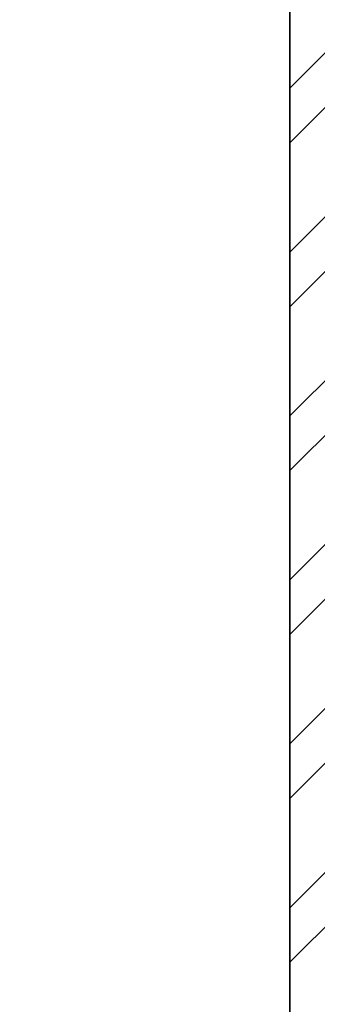
# Model space of a CAD drawing. Units: inches. Extents: x 2168 to 3056, y 1130 to 2629.
# Tile 30 of 42: x 2574 to 2598, y 2305 to 2386. Entities that reach past the tile are written whole.
import ezdxf

# ---------------------------------------------------------------- set-up
doc = ezdxf.new("R2010")
doc.units = ezdxf.units.IN
doc.layers.add('A-WALL', color=7, linetype='Continuous', lineweight=35)
doc.layers.add('A-WALL-PATT', color=143, linetype='Continuous', lineweight=13, true_color=0x7aafdf)

msp = doc.modelspace()

# ---------------------------------------------------------------- hatches: boundary and pattern name
at = {"layer": 'A-WALL-PATT'}
h = msp.add_hatch(dxfattribs=at)
h.set_pattern_fill('ANSI32', color=256)
h.paths.add_polyline_path([(2463.796, 2409.389), (2467.387, 2409.389), (2467.387, 2413.889), (2454.768, 2413.889), (2454.768, 2411.639), (2454.768, 2409.389), (2459.296, 2409.389), (2459.296, 2265.389), (2455.644, 2265.389), (2455.644, 2260.889), (2467.349, 2260.889), (2467.349, 2263.139), (2467.349, 2265.389), (2463.796, 2265.389)])
h.paths.add_polyline_path([(2431.596, 2413.889), (2409.647, 2413.889), (2409.647, 2409.389), (2431.596, 2409.389), (2431.596, 2411.639)])
h.paths.add_polyline_path([(2349.647, 2413.889), (2331.796, 2413.889), (2331.796, 2362.671), (2336.296, 2362.671), (2336.296, 2409.389), (2349.647, 2409.389), (2349.647, 2411.639)])
h.paths.add_polyline_path([(2634.149, 2411.639), (2634.149, 2413.889), (2562.293, 2413.889), (2562.293, 2409.389), (2595.796, 2409.389), (2595.796, 2280.309), (2595.826, 2280.309), (2595.826, 2265.389), (2499.91, 2265.389), (2499.91, 2260.889), (2550.796, 2260.889), (2550.796, 2117.308), (2555.296, 2117.308), (2555.296, 2168.08), (2571.93, 2168.08), (2571.93, 2176.889), (2559.796, 2176.889), (2559.796, 2256.389), (2640.796, 2256.389), (2640.796, 2176.889), (2626.428, 2176.889), (2626.428, 2168.08), (2645.296, 2168.08), (2645.296, 2116.637), (2649.796, 2116.637), (2649.796, 2260.889), (2691.251, 2260.889), (2691.251, 2263.139), (2691.251, 2265.389), (2670.655, 2265.389), (2670.655, 2265.365), (2600.296, 2265.365), (2600.296, 2280.258), (2600.296, 2409.389), (2634.149, 2409.389)])
h.paths.add_polyline_path([(2600.296, 2473.889), (2612.84, 2473.889), (2612.84, 2478.389), (2572.636, 2478.389), (2572.636, 2473.889), (2595.796, 2473.889), (2595.796, 2413.889), (2600.296, 2413.889)])
h.paths.add_polyline_path([(2535.796, 2473.889), (2548.636, 2473.889), (2548.636, 2478.389), (2531.396, 2478.389), (2531.396, 2413.889), (2521.6, 2413.889), (2521.6, 2409.389), (2539.239, 2409.389), (2539.239, 2411.639), (2539.239, 2413.889), (2535.796, 2413.889)])
h.paths.add_polyline_path([(2664.796, 2478.389), (2636.84, 2478.389), (2636.84, 2473.889), (2660.296, 2473.889), (2660.296, 2413.889), (2656.165, 2413.889), (2656.165, 2409.389), (2671.684, 2409.389), (2671.684, 2411.639), (2671.684, 2413.889), (2664.796, 2413.889)])
h.paths.add_polyline_path([(2705.942, 2413.889), (2695.684, 2413.889), (2695.684, 2409.389), (2705.942, 2409.389)])
h.paths.add_polyline_path([(2741.35, 2413.889), (2728.733, 2413.889), (2728.733, 2411.639), (2728.733, 2409.389), (2732.296, 2409.389), (2732.296, 2265.389), (2725.733, 2265.389), (2725.733, 2260.889), (2740.917, 2260.889), (2740.917, 2263.139), (2740.917, 2265.389), (2736.796, 2265.389), (2736.796, 2409.389), (2741.35, 2409.389)])
h.paths.add_polyline_path([(2785.655, 2413.889), (2764.546, 2413.889), (2764.486, 2409.389), (2785.655, 2409.389), (2785.655, 2411.639)])
h.paths.add_polyline_path([(2864.296, 2413.889), (2845.655, 2413.889), (2845.655, 2409.389), (2859.796, 2409.389), (2859.796, 2368.425), (2864.296, 2368.425)])
h.paths.add_polyline_path([(2864.296, 2308.425), (2862.046, 2308.425), (2859.796, 2308.425), (2859.796, 2265.389), (2774.483, 2265.389), (2774.483, 2263.139), (2774.483, 2260.889), (2781.796, 2260.889), (2781.796, 2226.654), (2786.296, 2226.654), (2786.296, 2260.889), (2859.796, 2260.889), (2859.796, 2241.352), (2864.296, 2241.352)])
h.paths.add_polyline_path([(2864.296, 2217.352), (2862.046, 2217.352), (2859.796, 2217.352), (2859.796, 2200.889), (2786.296, 2200.889), (2786.296, 2205.931), (2784.046, 2205.931), (2781.796, 2205.931), (2781.796, 2150.974), (2786.296, 2150.974), (2786.296, 2161.889), (2859.796, 2161.889), (2859.796, 2144.419), (2864.296, 2144.419)])
h.paths.add_polyline_path([(2859.796, 2196.389), (2859.796, 2166.389), (2786.296, 2166.389), (2786.296, 2196.389)], flags=16)
h.paths.add_polyline_path([(2864.296, 2108.419), (2862.046, 2108.419), (2859.796, 2108.419), (2859.796, 2080.889), (2786.296, 2080.889), (2786.296, 2111.993), (2781.796, 2111.993), (2781.796, 2080.889), (2649.796, 2080.889), (2649.796, 2086.036), (2647.546, 2086.036), (2645.296, 2086.036), (2645.296, 2071.739), (2649.796, 2071.739), (2649.796, 2076.389), (2781.796, 2076.389), (2781.796, 2041.792), (2786.296, 2041.792), (2786.296, 2076.389), (2859.796, 2076.389), (2859.796, 2058.577), (2864.296, 2058.577)])
h.paths.add_polyline_path([(2864.296, 2022.577), (2859.796, 2022.577), (2859.796, 1992.389), (2786.296, 1992.389), (2786.296, 1999.573), (2781.796, 1999.573), (2781.796, 1848.085), (2784.046, 1848.085), (2786.296, 1848.085), (2786.296, 1851.389), (2859.796, 1851.389), (2859.796, 1838.258), (2864.296, 1838.258)], flags=17)
h.paths.add_polyline_path([(2859.796, 1987.889), (2859.796, 1855.889), (2786.296, 1855.889), (2786.296, 1987.889)], flags=16)
h.paths.add_polyline_path([(2823.046, 1987.889), (2841.421, 1921.889), (2823.046, 1855.889)], flags=0)
h.paths.add_polyline_path([(2864.296, 1814.258), (2859.796, 1814.258), (2859.796, 1791.389), (2786.296, 1791.389), (2786.296, 1825.658), (2784.046, 1825.658), (2781.796, 1825.658), (2781.796, 1791.389), (2720.155, 1791.389), (2720.155, 1791.265), (2649.796, 1791.265), (2649.796, 1806.159), (2649.796, 2038.983), (2647.546, 2038.983), (2645.296, 2038.983), (2645.296, 1783.925), (2649.796, 1783.925), (2649.796, 1786.889), (2781.796, 1786.889), (2781.796, 1746.789), (2786.296, 1746.789), (2786.296, 1786.889), (2859.796, 1786.889), (2859.796, 1770.083), (2864.296, 1770.083)])
h.paths.add_polyline_path([(2864.296, 1734.083), (2862.046, 1734.083), (2859.796, 1734.083), (2859.796, 1705.889), (2786.296, 1705.889), (2786.296, 1714.166), (2781.796, 1714.166), (2781.796, 1660.527), (2786.296, 1660.527), (2786.296, 1666.889), (2859.796, 1666.889), (2859.796, 1648.342), (2864.296, 1648.342)])
h.paths.add_polyline_path([(2786.296, 1701.389), (2859.796, 1701.389), (2859.796, 1671.389), (2786.296, 1671.389)], flags=16)
h.paths.add_polyline_path([(2649.796, 1756.576), (2647.546, 1756.576), (2645.296, 1756.576), (2645.296, 1606.889), (2555.296, 1606.889), (2555.296, 1749.513), (2553.046, 1749.513), (2550.796, 1749.513), (2550.796, 1606.889), (2503.006, 1606.889), (2503.006, 1604.639), (2503.006, 1602.389), (2595.796, 1602.389), (2595.849, 1602.389), (2595.849, 1587.495), (2595.796, 1458.389), (2561.502, 1458.389), (2561.502, 1456.139), (2561.502, 1453.889), (2595.796, 1453.889), (2595.796, 1381.889), (2573.438, 1381.889), (2573.438, 1377.389), (2613.01, 1377.389), (2613.01, 1379.639), (2613.01, 1381.889), (2600.296, 1381.889), (2600.296, 1453.889), (2634.327, 1453.889), (2634.327, 1458.389), (2600.296, 1458.389), (2600.296, 1602.389), (2670.655, 1602.389), (2694.095, 1602.389), (2694.095, 1606.889), (2649.796, 1606.889)])
h.paths.add_polyline_path([(2736.796, 1602.389), (2741.562, 1602.389), (2741.562, 1606.889), (2726.203, 1606.889), (2726.203, 1604.639), (2726.203, 1602.389), (2732.296, 1602.389), (2732.296, 1458.389), (2727.899, 1458.389), (2727.899, 1453.889), (2740.821, 1453.889), (2740.821, 1456.139), (2740.821, 1458.389), (2736.796, 1458.389)])
h.paths.add_polyline_path([(2859.796, 1606.889), (2786.296, 1606.889), (2786.296, 1637.334), (2784.046, 1637.334), (2781.796, 1637.334), (2781.796, 1606.889), (2775.612, 1606.889), (2775.612, 1602.389), (2859.796, 1602.389)])
h.paths.add_polyline_path([(2864.296, 1624.342), (2862.046, 1624.342), (2859.796, 1624.342), (2859.796, 1570.39), (2864.296, 1570.39)])
h.paths.add_polyline_path([(2864.296, 1510.39), (2862.046, 1510.39), (2859.796, 1510.39), (2859.796, 1458.389), (2846.735, 1458.389), (2846.735, 1456.139), (2846.735, 1453.889), (2864.296, 1453.889)])
h.paths.add_polyline_path([(2786.735, 1458.389), (2765.444, 1458.389), (2765.444, 1453.889), (2786.735, 1453.889)])
h.paths.add_polyline_path([(2706.004, 1458.389), (2695.36, 1458.389), (2695.36, 1453.889), (2706.004, 1453.889), (2706.004, 1456.139)])
h.paths.add_polyline_path([(2671.36, 1456.139), (2671.36, 1458.389), (2655.986, 1458.389), (2655.986, 1456.139), (2655.986, 1453.889), (2660.296, 1453.889), (2660.296, 1381.889), (2637.01, 1381.889), (2637.01, 1377.389), (2664.796, 1377.389), (2664.796, 1453.889), (2671.36, 1453.889)], flags=17)
h.paths.add_polyline_path([(2539.829, 1458.389), (2520.237, 1458.389), (2520.237, 1453.889), (2531.296, 1453.889), (2531.296, 1377.389), (2546.449, 1377.389), (2546.449, 1379.639), (2546.449, 1381.889), (2535.796, 1381.889), (2535.796, 1453.889), (2539.829, 1453.889)], flags=17)
h.paths.add_polyline_path([(2496.237, 1458.389), (2489.13, 1458.389), (2489.13, 1453.889), (2496.237, 1453.889), (2496.237, 1456.139)])
h.paths.add_polyline_path([(2467.433, 1456.139), (2467.433, 1458.389), (2463.796, 1458.389), (2463.796, 1602.389), (2468.242, 1602.389), (2468.242, 1605.7), (2468.242, 1606.889), (2454.602, 1606.889), (2454.602, 1602.389), (2459.296, 1602.389), (2459.296, 1458.389), (2454.24, 1458.389), (2454.24, 1453.889), (2467.433, 1453.889)])
h.paths.add_polyline_path([(2431.601, 1456.139), (2431.601, 1458.389), (2411.386, 1458.389), (2411.386, 1453.889), (2431.601, 1453.889)])
h.paths.add_polyline_path([(2351.386, 1458.389), (2336.296, 1458.389), (2336.296, 1490.693), (2334.046, 1490.693), (2331.796, 1490.693), (2331.796, 1453.889), (2351.386, 1453.889), (2351.386, 1456.139)])
h.paths.add_polyline_path([(2336.296, 1629.705), (2331.796, 1629.705), (2331.796, 1552.317), (2336.296, 1552.317), (2336.296, 1602.389), (2406.655, 1602.389), (2423.472, 1602.389), (2423.472, 1606.889), (2418.796, 1606.889), (2418.796, 1643.678), (2416.546, 1643.678), (2414.296, 1643.678), (2414.296, 1606.889), (2336.296, 1606.889)])
h.paths.add_polyline_path([(2418.796, 1714.384), (2414.296, 1714.384), (2414.296, 1705.889), (2336.296, 1705.889), (2336.296, 1731.324), (2334.046, 1731.324), (2331.796, 1731.324), (2331.796, 1653.705), (2334.046, 1653.705), (2336.296, 1653.705), (2336.296, 1666.889), (2414.296, 1666.889), (2414.296, 1663.589), (2418.796, 1663.589)])
h.paths.add_polyline_path([(2336.296, 1701.389), (2414.296, 1701.389), (2414.296, 1671.389), (2336.296, 1671.389)], flags=16)
h.paths.add_polyline_path([(2555.296, 2040.059), (2550.796, 2040.059), (2550.796, 1791.389), (2550.561, 1791.205), (2480.202, 1791.205), (2418.796, 1791.389), (2418.796, 1825.448), (2416.546, 1825.448), (2414.296, 1825.448), (2414.296, 1791.389), (2336.296, 1791.389), (2336.296, 1806.409), (2331.796, 1806.409), (2331.796, 1767.324), (2336.296, 1767.324), (2336.296, 1786.889), (2414.296, 1786.889), (2414.296, 1745.457), (2418.796, 1745.457), (2418.796, 1786.889), (2550.796, 1786.889), (2550.796, 1783.011), (2555.296, 1783.011)])
h.paths.add_polyline_path([(2418.796, 1923.389), (2423.207, 1923.389), (2423.207, 1925.639), (2423.207, 1927.889), (2418.796, 1927.889), (2418.796, 2000.048), (2414.296, 2000.048), (2414.296, 1992.389), (2336.296, 1992.389), (2336.296, 1987.889), (2414.296, 1987.889), (2414.296, 1855.889), (2336.296, 1855.889), (2336.296, 1851.389), (2414.296, 1851.389), (2414.296, 1846.759), (2418.796, 1846.759)], flags=17)
h.paths.add_polyline_path([(2336.296, 2019.294), (2334.046, 2019.294), (2331.796, 2019.294), (2331.796, 1830.409), (2336.296, 1830.409)], flags=17)
h.paths.add_polyline_path([(2550.796, 1927.889), (2453.541, 1927.889), (2453.541, 1925.639), (2453.541, 1923.389), (2550.796, 1923.389)], flags=17)
h.paths.add_polyline_path([(2744.987, 1927.889), (2649.796, 1927.889), (2649.796, 1923.389), (2744.987, 1923.389), (2744.987, 1925.639)], flags=17)
h.paths.add_polyline_path([(2555.296, 2086.458), (2553.046, 2086.458), (2550.796, 2086.458), (2550.796, 2080.889), (2418.796, 2080.889), (2336.296, 2080.889), (2336.296, 2115.399), (2334.046, 2115.399), (2331.796, 2115.399), (2331.796, 2055.294), (2336.296, 2055.294), (2336.296, 2076.389), (2550.796, 2076.389), (2550.796, 2071.538), (2555.296, 2071.538)])
h.paths.add_polyline_path([(2418.796, 2121.389), (2414.296, 2121.389), (2414.296, 2080.889), (2418.796, 2080.889)])
h.paths.add_polyline_path([(2418.796, 2076.389), (2414.296, 2076.389), (2414.296, 2035.123), (2418.796, 2035.123)])
h.paths.add_polyline_path([(2422.868, 2263.139), (2422.868, 2265.389), (2406.655, 2265.389), (2406.655, 2265.359), (2336.296, 2265.359), (2336.296, 2280.252), (2336.296, 2302.671), (2334.046, 2302.671), (2331.796, 2302.671), (2331.796, 2246.853), (2336.296, 2246.853), (2336.296, 2260.889), (2414.296, 2260.889), (2414.296, 2223.996), (2418.796, 2223.996), (2418.796, 2260.889), (2422.868, 2260.889)])
h.paths.add_polyline_path([(2418.796, 2204.783), (2416.546, 2204.783), (2414.296, 2204.783), (2414.296, 2200.889), (2336.296, 2200.889), (2336.296, 2220.853), (2331.796, 2220.853), (2331.796, 2151.399), (2336.296, 2151.399), (2336.296, 2161.889), (2414.296, 2161.889), (2414.296, 2153.726), (2418.796, 2153.726)])
h.paths.add_polyline_path([(2414.296, 2196.389), (2414.296, 2166.389), (2336.296, 2166.389), (2336.296, 2196.389)], flags=16)
h.paths.add_polyline_path([(2375.296, 2181.389), (2336.296, 2166.389), (2336.296, 2196.389)], flags=0)
h.paths.add_polyline_path([(2809.595, 2172.34), (2838.804, 2172.34), (2838.804, 2190.997), (2809.595, 2190.997)], flags=8)
h.paths.add_polyline_path([(2849.75, 1919.585), (2849.75, 1952.672), (2831.093, 1952.672), (2831.093, 1919.585)], flags=8)
h.paths.add_polyline_path([(2808.875, 1901.967), (2808.875, 1937.85), (2790.149, 1937.85), (2790.149, 1901.967)], flags=8)
h.paths.add_polyline_path([(2806.285, 1671.896), (2835.493, 1671.896), (2835.493, 1690.553), (2806.285, 1690.553)], flags=8)
h.paths.add_polyline_path([(2353.186, 1676.549), (2382.395, 1676.549), (2382.395, 1695.207), (2353.186, 1695.207)], flags=8)
h.paths.add_polyline_path([(2360.083, 1832.308), (2389.241, 1832.308), (2389.241, 1850.966), (2360.083, 1850.966)], flags=25)
h.paths.add_polyline_path([(2354.822, 2167.823), (2384.031, 2167.823), (2384.031, 2186.481), (2354.822, 2186.481)], flags=8)

# ---------------------------------------------------------------- linework, layer by layer
at = {"layer": 'A-WALL'}
msp.add_line((2595.796, 2409.389), (2595.796, 2265.389), dxfattribs=at)

doc.saveas('drawing.dxf')
